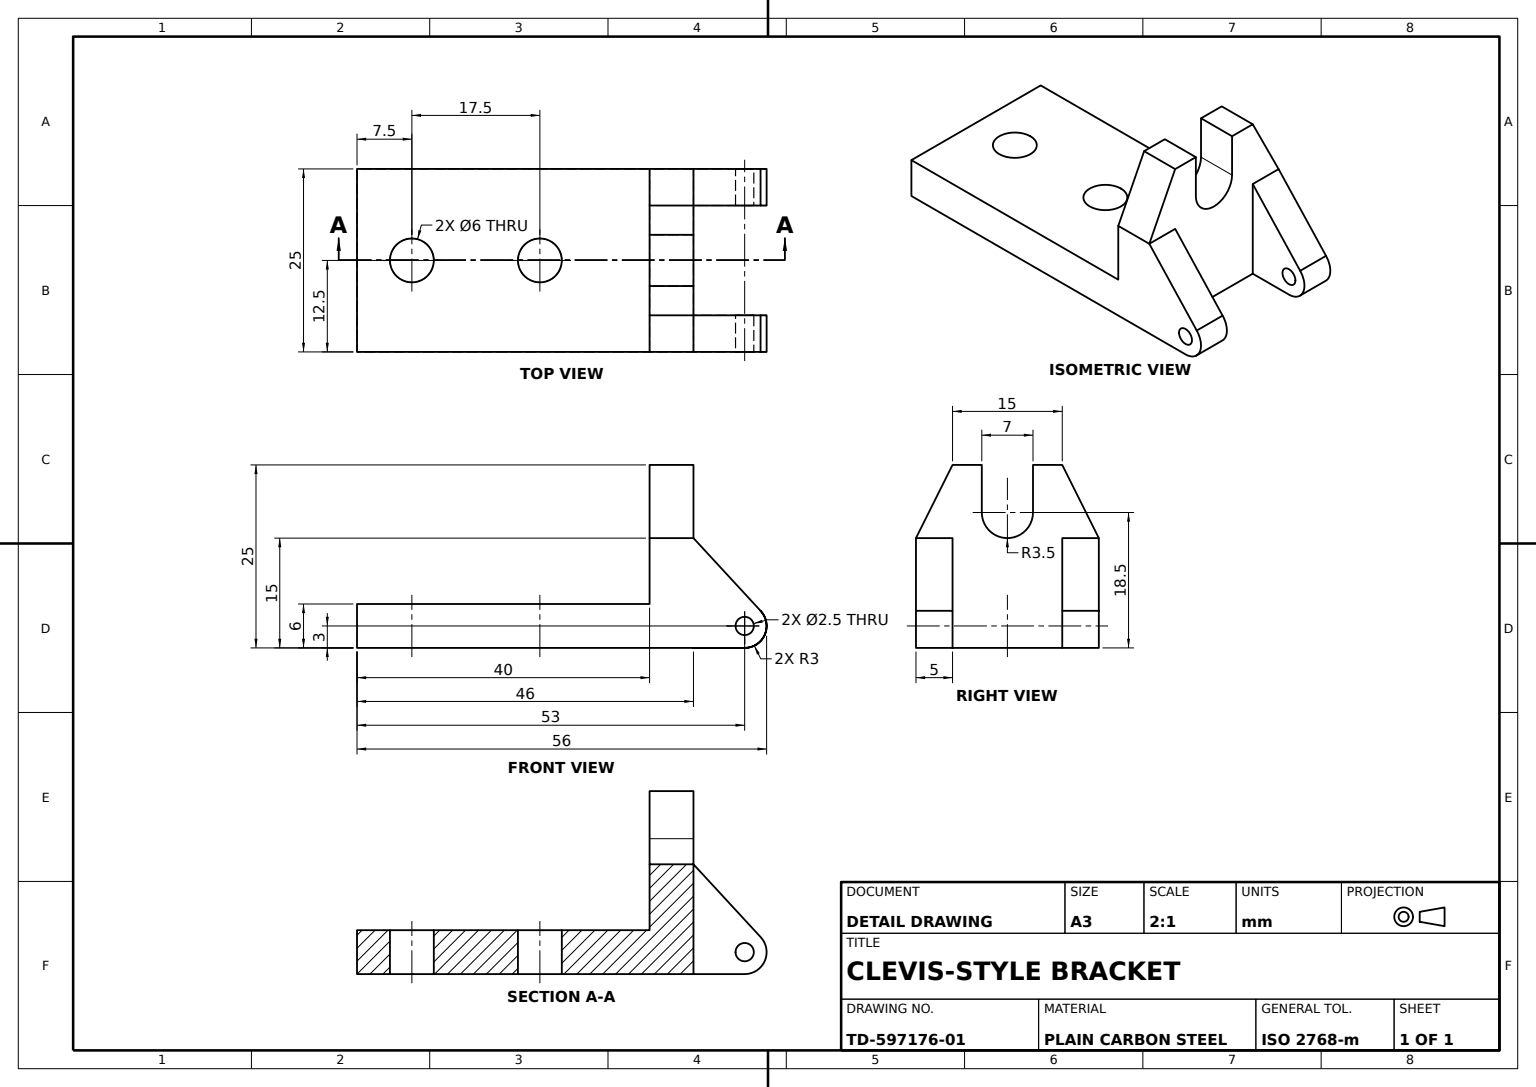
from build123d import *

# Parameters (mm, degrees)
BASE_PROFILE_SKETCH_W      = 40
BASE_PROFILE_SKETCH_H      = 6
BASE_BODY_DEPTH            = 25
UPRIGHT_BLOCK_SKETCH_W     = 6
UPRIGHT_BLOCK_SKETCH_H     = 15
UPRIGHT_BLOCK_DEPTH        = 25
SLOTTED_CLEVIS_PLATE_DEPTH = 6
LUG_1_DEPTH                = 5
LUG_1_PIN_HOLE_SKETCH_R    = 1.25
LUG_1_PIN_HOLE_DEPTH       = 5
LUG_START                  = -5
LUG_2_DEPTH                = 5
LUG_2_PIN_HOLE_SKETCH_R    = 1.25
LUG_2_PIN_HOLE_DEPTH       = 5
MOUNTING_HOLES_SKETCH_R    = 3
MOUNTING_HOLES_2X_6_DEPTH  = 6


with BuildPart() as part:
    # Base Profile Sketch → Base Body (new body)
    with BuildSketch(Plane.XY):
        with Locations((20, 3)):
            Rectangle(BASE_PROFILE_SKETCH_W, BASE_PROFILE_SKETCH_H)
    extrude(amount=BASE_BODY_DEPTH)

    # Upright Block Sketch → Upright Block (add)
    with BuildSketch(Plane.XY.offset(25)):
        with Locations((43, 7.5)):
            Rectangle(UPRIGHT_BLOCK_SKETCH_W, UPRIGHT_BLOCK_SKETCH_H)
    extrude(amount=-UPRIGHT_BLOCK_DEPTH)

    # Clevis Slot Profile Sketch → Slotted Clevis Plate (add)
    with BuildSketch(Plane.ZY.offset(-40)):
        with BuildLine():
            ThreePointArc((16, 18.5), (14.974873734, 16.025126266), (12.5, 15))
            Line((12.5, 15), (25, 15))
            Line((25, 15), (20, 25))
            Line((20, 25), (16, 25))
            Line((16, 25), (16, 18.5))
        make_face()
        with BuildLine():
            ThreePointArc((12.5, 15), (10.025126266, 16.025126266), (9, 18.5))
            Line((9, 18.5), (9, 25))
            Line((9, 25), (5, 25))
            Line((5, 25), (0, 15))
            Line((0, 15), (12.5, 15))
        make_face()
    extrude(amount=-SLOTTED_CLEVIS_PLATE_DEPTH)

    # Lug 1 Sketch → Lug 1 (add)
    with BuildSketch(Plane.XY.offset(25)):
        with BuildLine():
            Line((46, 0), (53, 0))
            ThreePointArc((53, 0), (55.757828687, 1.81916092), (55.171034593, 5.070412712))
            Line((55.171034593, 5.070412712), (46, 15))
            Line((46, 15), (46, 0))
        make_face()
    extrude(amount=-LUG_1_DEPTH)

    # Lug 1 Pin Hole Sketch → Lug 1 Pin Hole (cut)
    with BuildSketch(Plane.XY.offset(25)):
        with Locations((53, 3)):
            Circle(LUG_1_PIN_HOLE_SKETCH_R)
    extrude(amount=-LUG_1_PIN_HOLE_DEPTH, mode=Mode.SUBTRACT)

    # Lug 2 Sketch → Lug 2 (add)
    with BuildSketch(Plane(origin=(0, 0, 0), x_dir=(-1, 0, 0), z_dir=(0, 0, -1)).offset(LUG_START)):
        with BuildLine():
            Line((-46, 0), (-53, 0))
            ThreePointArc((-53, 0), (-55.757828687, 1.81916092), (-55.171034593, 5.070412712))
            Line((-55.171034593, 5.070412712), (-46, 15))
            Line((-46, 15), (-46, 0))
        make_face()
    extrude(amount=LUG_2_DEPTH)

    # Lug 2 Pin Hole Sketch → Lug 2 Pin Hole (cut)
    with BuildSketch(Plane(origin=(0, 0, 0), x_dir=(-1, 0, 0), z_dir=(0, 0, -1)).offset(LUG_START)):
        with Locations(Location((-53, 3, 0), (0, 0, 180))):
            Circle(LUG_2_PIN_HOLE_SKETCH_R)
    extrude(amount=LUG_2_PIN_HOLE_DEPTH, mode=Mode.SUBTRACT)

    # Mounting Holes Sketch → Mounting Holes 2xØ6 (cut)
    with BuildSketch(Plane(origin=(0, 6, 0), x_dir=(1, 0, 0), z_dir=(0, 1, 0))):
        with Locations(Location((7.5, -12.5, 0), (0, 0, 270))):
            Circle(MOUNTING_HOLES_SKETCH_R)
        with Locations(Location((25, -12.5, 0), (0, 0, 270))):
            Circle(MOUNTING_HOLES_SKETCH_R)
    extrude(amount=-MOUNTING_HOLES_2X_6_DEPTH, mode=Mode.SUBTRACT)


solid = part.part
